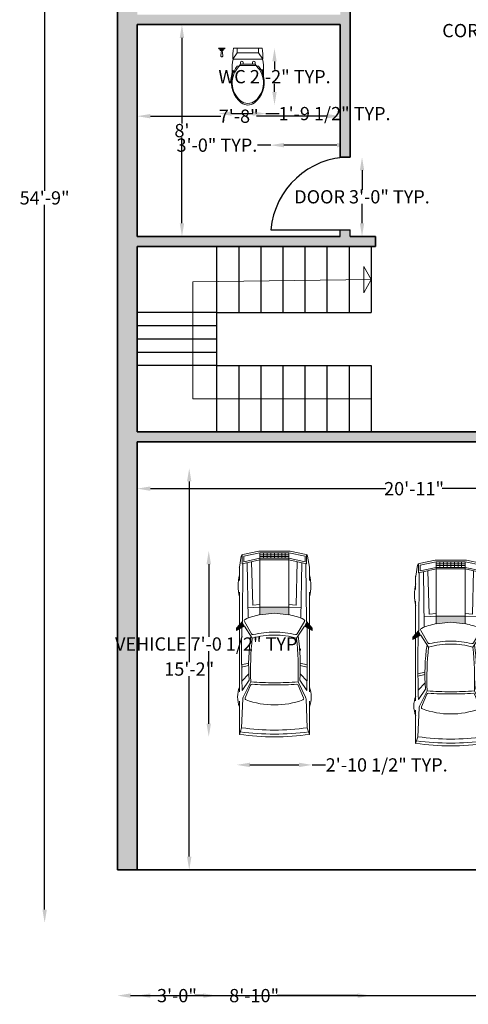
# Model space of a CAD drawing. Units: inches. Extents: x 2490 to 2996, y 1528 to 2269.
# Tile 1 of 4: x 2490 to 2693, y 1533 to 1979. Entities that reach past the tile are written whole.
import ezdxf

# ---------------------------------------------------------------- set-up
doc = ezdxf.new("R2010")
doc.units = ezdxf.units.IN
for name, color, linetype, lineweight in [('A-ANNO-DIMS', 2, 'Continuous', 18), ('A-DOOR', 4, 'Continuous', 25), ('A-EQPM-VEHL', 9, 'Continuous', 18), ('A-FLOR-STRS', 7, 'Continuous', 25), ('A-WALL', 7, 'Continuous', 35)]:
    doc.layers.add(name, color=color, linetype=linetype, lineweight=lineweight)
for name, color, linetype, lineweight, true_color in [('A-ANNO-SYMB', 244, 'Continuous', 18, 0x991b1e), ('A-FLOR-FIXT', 244, 'Continuous', 18, 0x991b1e), ('A-WALL-PATT', 85, 'Continuous', 13, 0x58ba48)]:
    doc.layers.add(name, color=color, linetype=linetype, lineweight=lineweight, true_color=true_color)
doc.styles.add('ATTR', font='romans.shx', dxfattribs={"width": 0.8, "height": 1.114828})
doc.styles.get("Standard").update_dxf_attribs({"font": 'arial.ttf'})
doc.dimstyles.get("Standard").update_dxf_attribs({"dimtxt": 6, "dimasz": 6, "dimexe": 0.18, "dimexo": 0.0625, "dimgap": 0.09, "dimtad": 0, "dimtih": 1, "dimtoh": 1, "dimdec": 4, "dimzin": 0, "dimdsep": 46, "dimlunit": 4, "dimtxsty": 'Standard', "dimcen": 0.09, "dimse1": 1, "dimse2": 1, "dimadec": 0, "dimazin": 0, "dimtfac": 1, "dimtdec": 4, "dimtofl": 0, "dimtmove": 0, "dimatfit": 3, "dimfxl": 1, "dimtolj": 1, "dimtzin": 0, "dimarcsym": 0})

# ---------------------------------------------------------------- blocks, each defined once
blk = doc.blocks.new('A$C682073C8')
for p, q in [((-2.78, 0.282), (-2.724, 0.571)), ((-2.69, 0.555), (-2.752, 0.263)), ((-2.554, 0.581), (-2.72, 0.581)), ((-2.694, 0.6), (-2.493, 0.633)), ((-2.59, 0.555), (-2.69, 0.555)), ((-2.59, 0.555), (-2.652, 0.263)), ((-2.554, 0.581), (-2.622, 0.263)), ((-2.557, 0.57), (-1.51, 0.58)), ((-2.251, 0.635), (-2.478, 0.635)), ((-1.445, 0.635), (-2.04, 0.635)), ((-1.51, 0.58), (-1.388, 0.684)), ((-1.286, 0.414), (-1.508, 0.544)), ((-1.428, 0.543), (-1.348, 0.684)), ((-1.209, 0.401), (-1.428, 0.543)), ((-1.388, 0.684), (-1.348, 0.684)), ((-0.237, 0.635), (-1.376, 0.635)), ((-0.755, 0.467), (-0.727, 0.593)), ((-0.714, 0.467), (-0.686, 0.593)), ((-0.432, 0.589), (-0.565, 0.464)), ((-0.451, 0.457), (-0.263, 0.585)), ((-0.142, 0.564), (-0.42, 0.428)), ((0.411, 0.593), (-0.11, 0.572)), ((0.532, 0.635), (-0.072, 0.635)), ((0.532, 0.635), (0.411, 0.593)), ((-1.805, 0.393), (-2.59, 0.413)), ((-1.57, 0.478), (-2.572, 0.496)), ((-1.818, 0.263), (-1.805, 0.393)), ((-1.771, 0.263), (-1.758, 0.481)), ((-0.361, 0.431), (-0.128, 0.528)), ((-2.781, 0), (-2.781, 0.273)), ((-2.752, 0.263), (-2.752, 0)), ((-1.633, 0.263), (-2.752, 0.263)), ((-2.652, 0.197), (-2.752, 0.197)), ((-2.718, 0.263), (-2.718, 0)), ((-2.685, 0.263), (-2.685, 0)), ((-2.652, 0.263), (-2.652, 0)), ((-2.622, 0.263), (-2.622, 0)), ((-1.771, 0.263), (-1.771, 0)), ((-1.633, 0.263), (-1.659, 0)), ((-2.781, 0), (-2.781, -0.273)), ((-2.652, 0.132), (-2.752, 0.132)), ((-2.652, 0.066), (-2.752, 0.066)), ((-2.652, 0), (-2.752, 0)), ((-2.752, -0.263), (-2.752, 0)), ((-2.718, -0.263), (-2.718, 0)), ((-2.685, -0.263), (-2.685, 0)), ((-2.652, -0.263), (-2.652, 0)), ((-2.622, -0.263), (-2.622, 0)), ((-1.771, -0.263), (-1.771, 0)), ((-1.659, 0), (-1.633, -0.263)), ((-2.652, -0.066), (-2.752, -0.066)), ((-2.652, -0.132), (-2.752, -0.132)), ((-2.78, -0.282), (-2.724, -0.571)), ((-2.652, -0.197), (-2.752, -0.197)), ((-1.633, -0.263), (-2.752, -0.263)), ((-2.69, -0.555), (-2.752, -0.263)), ((-2.59, -0.555), (-2.652, -0.263)), ((-2.554, -0.581), (-2.622, -0.263)), ((-1.818, -0.263), (-1.805, -0.393)), ((-1.771, -0.263), (-1.758, -0.481)), ((-1.805, -0.393), (-2.59, -0.413)), ((-1.57, -0.478), (-2.572, -0.496)), ((-1.286, -0.414), (-1.508, -0.544)), ((-1.209, -0.401), (-1.428, -0.543)), ((-0.755, -0.467), (-0.727, -0.593)), ((-0.714, -0.467), (-0.686, -0.593)), ((-0.432, -0.589), (-0.565, -0.464)), ((-0.451, -0.457), (-0.263, -0.585)), ((-0.142, -0.564), (-0.42, -0.428)), ((-0.361, -0.431), (-0.128, -0.528)), ((-2.554, -0.581), (-2.72, -0.581)), ((-2.694, -0.6), (-2.493, -0.633)), ((-2.59, -0.555), (-2.69, -0.555)), ((-2.557, -0.57), (-1.51, -0.58)), ((-2.251, -0.635), (-2.478, -0.635)), ((-1.445, -0.635), (-2.04, -0.635)), ((-1.51, -0.58), (-1.388, -0.684)), ((-1.428, -0.543), (-1.348, -0.684)), ((-1.388, -0.684), (-1.348, -0.684)), ((-0.237, -0.635), (-1.376, -0.635)), ((0.411, -0.593), (-0.11, -0.572)), ((0.532, -0.635), (-0.072, -0.635)), ((0.532, -0.635), (0.411, -0.593))]:
    blk.add_line(p, q)
for centre, radius, start, end in [((-2.688, 0.564), 0.0366, 99.5555, 168.9219), ((-2.478, 0.542), 0.0932, 90, 99.5555), ((-2.154, -0.189), 0.847, 76.4679, 103.5321), ((-1.522, 0.52), 0.0277, 59.6014, 156.2323), ((-0.97, -26.413), 27.007, 88.4985, 90.9138), ((-0.146, 0.162), 0.505, 69.2613, 110.7387), ((-0.106, 0.49), 0.0817, 92.3222, 116.0777), ((-3.642, 0), 4.096, 360, 8.3245), ((-4.512, 0), 5.038, 360, 7.0662), ((-3.75, 0), 4.328, 360, 8.4328), ((-0.341, 0), 1.319, 156.2323, 168.4871), ((0.324, 0), 1.642, 166.5017, 180), ((-1.3, 0.39), 0.0277, 346.5017, 59.6014), ((0.222, 0), 1.487, 164.3473, 180), ((-0.728, -3.189), 3.656, 85.6618, 98.2609), ((-0.642, -4.704), 5.136, 87.5218, 96.3432), ((-5.551, 0), 5.149, 360, 4.7655), ((-0.35, 0.407), 0.0264, 112.6283, 183.982), ((-6.195, 0), 5.833, 360, 3.982), ((-0.118, 0.504), 0.0264, 20.6689, 112.6283), ((-1.453, 0), 1.453, 360, 20.6689), ((-2.736, 0.273), 0.045, 168.9219, 180), ((0.324, 0), 1.642, 180, 193.4983), ((0.222, 0), 1.487, 180, 195.6527), ((-5.551, 0), 5.149, 355.2345, 360), ((-6.195, 0), 5.833, 356.018, 360), ((-1.453, 0), 1.453, 339.3311, 360), ((-3.642, 0), 4.096, 351.6755, 360), ((-4.512, 0), 5.038, 352.9338, 360), ((-3.75, 0), 4.328, 351.5672, 360), ((-2.736, -0.273), 0.045, 180, 191.0781), ((-0.341, 0), 1.319, 191.5129, 203.7677), ((-1.522, -0.52), 0.0277, 203.7677, 300.3986), ((-1.3, -0.39), 0.0277, 300.3986, 13.4983), ((-0.728, 3.189), 3.656, 261.7391, 274.3382), ((-0.642, 4.704), 5.136, 263.6568, 272.4781), ((-0.35, -0.407), 0.0264, 176.018, 247.3717), ((-0.118, -0.504), 0.0264, 247.3717, 339.3311), ((-2.688, -0.564), 0.0366, 191.0781, 260.4445), ((-2.478, -0.542), 0.0932, 260.4445, 270), ((-2.154, 0.189), 0.847, 256.4679, 283.5321), ((-0.97, 26.413), 27.007, 269.0862, 271.5015), ((-0.146, -0.162), 0.505, 249.2613, 290.7387), ((-0.106, -0.49), 0.0817, 243.9223, 267.6778)]:
    blk.add_arc(centre, radius, start, end)
for points in [[(-1.428, 0.543), (-1.51, 0.58), (-1.348, 0.684), (-1.388, 0.684)], [(-1.633, 0.263), (-1.659, 0), (-1.771, 0.263), (-1.771, -0.263)], [(-1.659, 0), (-1.633, -0.263), (-1.771, -0.263)], [(-1.428, -0.543), (-1.51, -0.58), (-1.348, -0.684), (-1.388, -0.684)]]:
    blk.add_solid(points)
at = {"style": 'ATTR', "width": 0.8, "flags": 9}
blk.add_attdef('ESTCODE', (-2.781, 0), '', height=0.00071, rotation=180, dxfattribs=at)
blk = doc.blocks.new('*D16')
at = {"layer": 'A-ANNO-DIMS', "color": 0, "lineweight": -2, "transparency": 16777216}
for p, q in [((2563.55, 1971.13), (2563.55, 1932.29)), ((2563.55, 1887.13), (2563.55, 1925.98))]:
    blk.add_line(p, q, dxfattribs=at)
at = {"layer": 'A-ANNO-DIMS', "color": 0, "transparency": 16777216}
for points in [[(2562.55, 1971.13), (2564.55, 1971.13), (2563.55, 1977.13)], [(2562.55, 1887.13), (2564.55, 1887.13), (2563.55, 1881.13)]]:
    blk.add_solid(points, dxfattribs=at)
at = {"layer": 'Defpoints', "color": 0, "transparency": 16777216}
for p in [(2543.28, 1977.13), (2543.28, 1881.13), (2563.55, 1881.13)]:
    blk.add_point(p, dxfattribs=at)
at = {"layer": 'A-ANNO-DIMS', "color": 0, "transparency": 16777216, "insert": (2563.55, 1929.13), "char_height": 6, "attachment_point": 5}
blk.add_mtext("\\A1;8'", dxfattribs=at)
blk = doc.blocks.new('*D17')
at = {"layer": 'A-ANNO-DIMS', "color": 0, "lineweight": -2, "transparency": 16777216}
for p, q in [((2549.28, 1935.65), (2581.24, 1935.65)), ((2629.28, 1935.65), (2597.32, 1935.65))]:
    blk.add_line(p, q, dxfattribs=at)
at = {"layer": 'A-ANNO-DIMS', "color": 0, "transparency": 16777216}
for points in [[(2549.28, 1936.65), (2549.28, 1934.65), (2543.28, 1935.65)], [(2629.28, 1936.65), (2629.28, 1934.65), (2635.28, 1935.65)]]:
    blk.add_solid(points, dxfattribs=at)
at = {"layer": 'Defpoints', "color": 0, "transparency": 16777216}
for p in [(2543.28, 1977.13), (2635.28, 1977.13), (2635.28, 1935.65)]:
    blk.add_point(p, dxfattribs=at)
at = {"layer": 'A-ANNO-DIMS', "color": 0, "transparency": 16777216, "insert": (2589.28, 1935.65), "char_height": 6, "attachment_point": 5}
blk.add_mtext('\\A1;7\'-8"', dxfattribs=at)
blk = doc.blocks.new('*D18')
at = {"layer": 'A-ANNO-DIMS', "color": 0, "lineweight": -2, "transparency": 16777216}
for p, q in [((2566.85, 1770.13), (2566.85, 1688.29)), ((2566.85, 1600.13), (2566.85, 1681.98))]:
    blk.add_line(p, q, dxfattribs=at)
at = {"layer": 'A-ANNO-DIMS', "color": 0, "transparency": 16777216}
for points in [[(2565.85, 1770.13), (2567.85, 1770.13), (2566.85, 1776.13)], [(2565.85, 1600.13), (2567.85, 1600.13), (2566.85, 1594.13)]]:
    blk.add_solid(points, dxfattribs=at)
at = {"layer": 'Defpoints', "color": 0, "transparency": 16777216}
for p in [(2543.28, 1776.13), (2543.28, 1594.13), (2566.85, 1594.13)]:
    blk.add_point(p, dxfattribs=at)
at = {"layer": 'A-ANNO-DIMS', "color": 0, "transparency": 16777216, "insert": (2566.85, 1685.13), "char_height": 6, "attachment_point": 5}
blk.add_mtext('\\A1;15\'-2"', dxfattribs=at)
blk = doc.blocks.new('*D19')
at = {"layer": 'A-ANNO-DIMS', "color": 0, "lineweight": -2, "transparency": 16777216}
for p, q in [((2549.28, 1766.88), (2656, 1766.88)), ((2788.28, 1766.88), (2681.56, 1766.88))]:
    blk.add_line(p, q, dxfattribs=at)
at = {"layer": 'A-ANNO-DIMS', "color": 0, "transparency": 16777216}
for points in [[(2549.28, 1767.88), (2549.28, 1765.88), (2543.28, 1766.88)], [(2788.28, 1767.88), (2788.28, 1765.88), (2794.28, 1766.88)]]:
    blk.add_solid(points, dxfattribs=at)
at = {"layer": 'Defpoints', "color": 0, "transparency": 16777216}
for p in [(2794.28, 1766.88), (2543.28, 1759.76), (2794.28, 1759.76)]:
    blk.add_point(p, dxfattribs=at)
at = {"layer": 'A-ANNO-DIMS', "color": 0, "transparency": 16777216, "insert": (2668.78, 1766.88), "char_height": 6, "attachment_point": 5}
blk.add_mtext('\\A1;20\'-11"', dxfattribs=at)
blk = doc.blocks.new('WC-PLAN')
for p, q in [((9.57, 17.88), (9.93, 18.54)), ((9.93, 18.54), (9.93, 19.26)), ((11.22, 18.54), (9.93, 18.54)), ((11.22, 19.26), (11.22, 18.54)), ((13.29, 18.54), (11.22, 18.54)), ((13.29, 18.54), (15.36, 18.54)), ((15.36, 19.26), (15.36, 18.54)), ((15.36, 18.54), (16.65, 18.54)), ((16.65, 18.54), (16.65, 19.26)), ((17.01, 17.88), (16.65, 18.54))]:
    blk.add_line(p, q)
for points in [[(2.96, 25.75), (0, 25.75)], [(2.78, 25.55), (0.18, 25.55)], [(2.16, 25.2), (0.8, 25.2)], [(0.8, 25.2), (0.8, 24.77), (1.28, 24.77)], [(1.15, 25.2), (1.15, 24.77)], [(1.28, 24.77), (1.71, 24.77)], [(1.71, 24.77), (2.14, 24.77), (2.16, 25.2)], [(1.84, 25.2), (1.84, 24.77)], [(6.49, 20.79), (8.51, 23.63), (8.51, 25.75)], [(19.81, 25.75), (6.76, 25.75)], [(8.51, 23.63), (13.29, 23.63)], [(18.06, 23.63), (13.29, 23.63)], [(20.09, 20.79), (18.06, 23.63), (18.06, 25.75)], [(6.61, 20.79), (13.29, 20.79)], [(19.96, 20.79), (13.29, 20.79)]]:
    blk.add_lwpolyline(points)
for points in [[(0.8, 25.2, -0.158381), (0, 25.75, 2.932383)], [(1.28, 24.75), (1.02, 22.39, 0.482607), (1.52, 21.9, -0.547905)], [(1.71, 24.75), (1.97, 22.39, -0.482607), (1.47, 21.9, 0.547905)], [(2.16, 25.2, 0.158381), (2.96, 25.75, -2.932383)], [(6.76, 25.75, 0.056711), (6.49, 20.79), (6.61, 20.79)], [(19.81, 25.75, -0.056711), (20.09, 20.79), (19.96, 20.79)], [(6.61, 20.78, 0.052121), (6.14, 15.38), (6.14, 13.01, 0.14456)], [(9.57, 17.88, 0.008985), (9.29, 17.61, 0.182634)], [(13.29, 17.88), (9.57, 17.88, 0.008985)], [(13.29, 17.88), (17.01, 17.88, -0.444938)], [(17.01, 17.88, -0.008985), (17.28, 17.61, -0.182634)], [(19.96, 20.78, -0.052121), (20.43, 15.38), (20.43, 13.01, -0.14456)], [(8.4, 17.61, 0.11024), (6.14, 13.01, 0.16845)], [(9.29, 17.61, 0.434217), (9.93, 1.97, 0.182634), (13.29, 0.75, 2.693815)], [(9.29, 17.61), (8.4, 17.61, 0.416606)], [(17.28, 17.61, -0.434217), (16.65, 1.97, -0.182634), (13.29, 0.75, -2.693815)], [(17.28, 17.61), (18.18, 17.61, -0.416606)], [(18.18, 17.61, -0.11024), (20.43, 13.01, -0.16845)], [(6.14, 13.01, 0.292914), (10.29, 1.04, 0.16845), (13.29, 0, 2.883082)], [(20.43, 13.01, -0.292914), (16.29, 1.04, -0.16845), (13.29, 0, -2.883082)]]:
    blk.add_lwpolyline(points, format="xyb")
for centre in [(10.57, 19.26), (16, 19.26)]:
    blk.add_arc(centre, 0.645, 0, 180)
blk = doc.blocks.new('DOOR-SINGLE-36IN')
for p, q in [((0, 36), (0, 4.5)), ((3, 35.88), (3, 0)), ((0, 4.5), (3, 4.5)), ((0, 0), (3, 0))]:
    blk.add_line(p, q)
blk.add_arc((0, 0), 36, 0, 85.2198)
blk = doc.blocks.new('*D32')
at = {"layer": 'A-ANNO-DIMS', "color": 0, "lineweight": -2, "transparency": 16777216}
for p, q in [((2605.51, 1960.45), (2605.51, 1956.76)), ((2605.51, 1946.69), (2605.51, 1950.38))]:
    blk.add_line(p, q, dxfattribs=at)
at = {"layer": 'A-ANNO-DIMS', "color": 0, "transparency": 16777216}
for points in [[(2604.51, 1960.45), (2606.51, 1960.45), (2605.51, 1966.45)], [(2604.51, 1946.69), (2606.51, 1946.69), (2605.51, 1940.69)]]:
    blk.add_solid(points, dxfattribs=at)
at = {"layer": 'Defpoints', "color": 0, "transparency": 16777216}
for p in [(2601.65, 1966.45), (2605.51, 1966.45), (2601.65, 1940.69)]:
    blk.add_point(p, dxfattribs=at)
at = {"layer": 'A-ANNO-DIMS', "color": 0, "transparency": 16777216, "insert": (2605.51, 1953.57), "char_height": 6, "attachment_point": 5}
blk.add_mtext('\\A1;WC 2\'-2" TYP.', dxfattribs=at)
blk = doc.blocks.new('*D33')
at = {"layer": 'A-ANNO-DIMS', "color": 0, "lineweight": -2, "transparency": 16777216}
for p, q in [((2586.14, 1936.83), (2595.65, 1936.83)), ((2601.65, 1936.83), (2607.65, 1936.83))]:
    blk.add_line(p, q, dxfattribs=at)
at = {"layer": 'A-ANNO-DIMS', "color": 0, "transparency": 16777216}
for points in [[(2586.14, 1937.83), (2586.14, 1935.83), (2580.14, 1936.83)], [(2595.65, 1937.83), (2595.65, 1935.83), (2601.65, 1936.83)]]:
    blk.add_solid(points, dxfattribs=at)
at = {"layer": 'Defpoints', "color": 0, "transparency": 16777216}
for p in [(2580.14, 1940.69), (2601.65, 1940.69), (2601.65, 1936.83)]:
    blk.add_point(p, dxfattribs=at)
at = {"layer": 'A-ANNO-DIMS', "color": 0, "transparency": 16777216, "insert": (2632.73, 1936.83), "char_height": 6, "attachment_point": 5}
blk.add_mtext('\\A1;1\'-9 1/2" TYP.', dxfattribs=at)
blk = doc.blocks.new('*D34')
at = {"layer": 'A-ANNO-DIMS', "color": 0, "lineweight": -2, "transparency": 16777216}
for p, q in [((2645.18, 1911.13), (2645.18, 1902.33)), ((2645.18, 1887.13), (2645.18, 1895.94))]:
    blk.add_line(p, q, dxfattribs=at)
at = {"layer": 'A-ANNO-DIMS', "color": 0, "transparency": 16777216}
for points in [[(2644.18, 1911.13), (2646.18, 1911.13), (2645.18, 1917.13)], [(2644.18, 1887.13), (2646.18, 1887.13), (2645.18, 1881.13)]]:
    blk.add_solid(points, dxfattribs=at)
at = {"layer": 'Defpoints', "color": 0, "transparency": 16777216}
for p in [(2639.78, 1917.13), (2645.18, 1917.13), (2639.78, 1881.13)]:
    blk.add_point(p, dxfattribs=at)
at = {"layer": 'A-ANNO-DIMS', "color": 0, "transparency": 16777216, "insert": (2645.18, 1899.13), "char_height": 6, "attachment_point": 5}
blk.add_mtext('\\A1;DOOR 3\'-0" TYP.', dxfattribs=at)
blk = doc.blocks.new('*D35')
at = {"layer": 'A-ANNO-DIMS', "color": 0, "lineweight": -2, "transparency": 16777216}
for p, q in [((2603.78, 1922.53), (2597.78, 1922.53)), ((2633.78, 1922.53), (2609.78, 1922.53))]:
    blk.add_line(p, q, dxfattribs=at)
at = {"layer": 'A-ANNO-DIMS', "color": 0, "transparency": 16777216}
for points in [[(2609.78, 1923.53), (2609.78, 1921.53), (2603.78, 1922.53)], [(2633.78, 1923.53), (2633.78, 1921.53), (2639.78, 1922.53)]]:
    blk.add_solid(points, dxfattribs=at)
at = {"layer": 'Defpoints', "color": 0, "transparency": 16777216}
for p in [(2603.78, 1922.53), (2603.78, 1917.13), (2639.78, 1917.13)]:
    blk.add_point(p, dxfattribs=at)
at = {"layer": 'A-ANNO-DIMS', "color": 0, "transparency": 16777216, "insert": (2579.4, 1922.53), "char_height": 6, "attachment_point": 5}
blk.add_mtext('\\A1;3\'-0" TYP.', dxfattribs=at)
blk = doc.blocks.new('*D38')
at = {"layer": 'A-ANNO-DIMS', "color": 0, "lineweight": -2, "transparency": 16777216}
for p, q in [((2575.7, 1732.64), (2575.7, 1699.69)), ((2575.7, 1660.35), (2575.7, 1693.3))]:
    blk.add_line(p, q, dxfattribs=at)
at = {"layer": 'A-ANNO-DIMS', "color": 0, "transparency": 16777216}
for points in [[(2574.7, 1732.64), (2576.7, 1732.64), (2575.7, 1738.64)], [(2574.7, 1660.35), (2576.7, 1660.35), (2575.7, 1654.35)]]:
    blk.add_solid(points, dxfattribs=at)
at = {"layer": 'Defpoints', "color": 0, "transparency": 16777216}
for p in [(2588.35, 1738.64), (2575.7, 1654.35), (2588.35, 1654.35)]:
    blk.add_point(p, dxfattribs=at)
at = {"layer": 'A-ANNO-DIMS', "color": 0, "transparency": 16777216, "insert": (2575.7, 1696.49), "char_height": 6, "attachment_point": 5}
blk.add_mtext('\\A1;VEHICLE 7\'-0 1/2" TYP.', dxfattribs=at)
blk = doc.blocks.new('*D39')
at = {"layer": 'A-ANNO-DIMS', "color": 0, "lineweight": -2, "transparency": 16777216}
for p, q in [((2594.35, 1641.7), (2616.61, 1641.7)), ((2622.61, 1641.7), (2628.61, 1641.7))]:
    blk.add_line(p, q, dxfattribs=at)
at = {"layer": 'A-ANNO-DIMS', "color": 0, "transparency": 16777216}
for points in [[(2594.35, 1642.7), (2594.35, 1640.7), (2588.35, 1641.7)], [(2616.61, 1642.7), (2616.61, 1640.7), (2622.61, 1641.7)]]:
    blk.add_solid(points, dxfattribs=at)
at = {"layer": 'Defpoints', "color": 0, "transparency": 16777216}
for p in [(2588.35, 1654.35), (2622.61, 1654.35), (2622.61, 1641.7)]:
    blk.add_point(p, dxfattribs=at)
at = {"layer": 'A-ANNO-DIMS', "color": 0, "transparency": 16777216, "insert": (2656.36, 1641.7), "char_height": 6, "attachment_point": 5}
blk.add_mtext('\\A1;2\'-10 1/2" TYP.', dxfattribs=at)
blk = doc.blocks.new('*D40')
at = {"layer": 'A-ANNO-DIMS', "color": 0, "lineweight": -2, "transparency": 16777216}
for p, q in [((2801.71, 1974.44), (2795.71, 1974.44)), ((2821.13, 1974.44), (2807.71, 1974.44))]:
    blk.add_line(p, q, dxfattribs=at)
at = {"layer": 'A-ANNO-DIMS', "color": 0, "transparency": 16777216}
for points in [[(2807.71, 1975.44), (2807.71, 1973.44), (2801.71, 1974.44)], [(2821.13, 1975.44), (2821.13, 1973.44), (2827.13, 1974.44)]]:
    blk.add_solid(points, dxfattribs=at)
at = {"layer": 'Defpoints', "color": 0, "transparency": 16777216}
for p in [(2801.71, 1974.44), (2801.71, 1970.63), (2827.13, 1970.63)]:
    blk.add_point(p, dxfattribs=at)
at = {"layer": 'A-ANNO-DIMS', "color": 0, "transparency": 16777216, "insert": (2736.85, 1974.44), "char_height": 6, "attachment_point": 5}
blk.add_mtext('\\A1;CORNER CHAIR 2\'-1 1/2" TYP.', dxfattribs=at)
blk = doc.blocks.new('*D46')
at = {"layer": 'A-ANNO-DIMS', "color": 0, "lineweight": -2, "transparency": 16777216}
for p, q in [((2540.28, 1537.16), (2732.39, 1537.16)), ((2945.28, 1537.16), (2753.17, 1537.16))]:
    blk.add_line(p, q, dxfattribs=at)
at = {"layer": 'A-ANNO-DIMS', "color": 0, "transparency": 16777216}
for points in [[(2540.28, 1538.16), (2540.28, 1536.16), (2534.28, 1537.16)], [(2945.28, 1538.16), (2945.28, 1536.16), (2951.28, 1537.16)]]:
    blk.add_solid(points, dxfattribs=at)
at = {"layer": 'Defpoints', "color": 0, "transparency": 16777216}
for p in [(2951.28, 1600.13), (2534.28, 1594.13), (2951.28, 1537.16)]:
    blk.add_point(p, dxfattribs=at)
at = {"layer": 'A-ANNO-DIMS', "color": 0, "transparency": 16777216, "insert": (2742.78, 1537.16), "char_height": 6, "attachment_point": 5}
blk.add_mtext('\\A1;34\'-9"', dxfattribs=at)
blk = doc.blocks.new('*D47')
at = {"layer": 'A-ANNO-DIMS', "color": 0, "lineweight": -2, "transparency": 16777216}
for p, q in [((2501.3, 2221.13), (2501.3, 1901.79)), ((2501.3, 1576.13), (2501.3, 1895.48))]:
    blk.add_line(p, q, dxfattribs=at)
at = {"layer": 'A-ANNO-DIMS', "color": 0, "transparency": 16777216}
for points in [[(2500.3, 2221.13), (2502.3, 2221.13), (2501.3, 2227.13)], [(2500.3, 1576.13), (2502.3, 1576.13), (2501.3, 1570.13)]]:
    blk.add_solid(points, dxfattribs=at)
at = {"layer": 'Defpoints', "color": 0, "transparency": 16777216}
for p in [(2501.3, 2227.13), (2534.28, 2227.13), (2758.28, 1570.13)]:
    blk.add_point(p, dxfattribs=at)
at = {"layer": 'A-ANNO-DIMS', "color": 0, "transparency": 16777216, "insert": (2501.3, 1898.63), "char_height": 6, "attachment_point": 5}
blk.add_mtext('\\A1;54\'-9"', dxfattribs=at)
blk = doc.blocks.new('*D50')
at = {"layer": 'A-ANNO-DIMS', "color": 0, "lineweight": -2, "transparency": 16777216}
for p, q in [((2984.25, 1870.63), (2984.25, 1837.79)), ((2984.25, 1798.63), (2984.25, 1831.48))]:
    blk.add_line(p, q, dxfattribs=at)
at = {"layer": 'A-ANNO-DIMS', "color": 0, "transparency": 16777216}
for points in [[(2983.25, 1870.63), (2985.25, 1870.63), (2984.25, 1876.63)], [(2983.25, 1798.63), (2985.25, 1798.63), (2984.25, 1792.63)]]:
    blk.add_solid(points, dxfattribs=at)
at = {"layer": 'Defpoints', "color": 0, "transparency": 16777216}
for p in [(2649.28, 1876.63), (2984.25, 1876.63), (2649.28, 1792.63)]:
    blk.add_point(p, dxfattribs=at)
at = {"layer": 'A-ANNO-DIMS', "color": 0, "transparency": 16777216, "insert": (2984.25, 1834.63), "char_height": 6, "attachment_point": 5}
blk.add_mtext('\\A1;7\'-0"', dxfattribs=at)
blk = doc.blocks.new('*D51')
at = {"layer": 'A-ANNO-DIMS', "color": 0, "lineweight": -2, "transparency": 16777216}
for p, q in [((2549.28, 1537.16), (2585.88, 1537.16)), ((2643.28, 1537.16), (2606.68, 1537.16))]:
    blk.add_line(p, q, dxfattribs=at)
at = {"layer": 'A-ANNO-DIMS', "color": 0, "transparency": 16777216}
for points in [[(2549.28, 1538.16), (2549.28, 1536.16), (2543.28, 1537.16)], [(2643.28, 1538.16), (2643.28, 1536.16), (2649.28, 1537.16)]]:
    blk.add_solid(points, dxfattribs=at)
at = {"layer": 'Defpoints', "color": 0, "transparency": 16777216}
for p in [(2543.28, 1792.63), (2649.28, 1792.63), (2649.28, 1537.16)]:
    blk.add_point(p, dxfattribs=at)
at = {"layer": 'A-ANNO-DIMS', "color": 0, "transparency": 16777216, "insert": (2596.28, 1537.16), "char_height": 6, "attachment_point": 5}
blk.add_mtext('\\A1;8\'-10"', dxfattribs=at)
blk = doc.blocks.new('*D52')
at = {"layer": 'A-ANNO-DIMS', "color": 0, "lineweight": -2, "transparency": 16777216}
for p, q in [((2984.25, 1816.63), (2984.25, 1810.79)), ((2984.25, 1798.63), (2984.25, 1804.48))]:
    blk.add_line(p, q, dxfattribs=at)
at = {"layer": 'A-ANNO-DIMS', "color": 0, "transparency": 16777216}
for points in [[(2983.25, 1816.63), (2985.25, 1816.63), (2984.25, 1822.63)], [(2983.25, 1798.63), (2985.25, 1798.63), (2984.25, 1792.63)]]:
    blk.add_solid(points, dxfattribs=at)
at = {"layer": 'Defpoints', "color": 0, "transparency": 16777216}
for p in [(2649.28, 1822.63), (2984.25, 1822.63), (2649.28, 1792.63)]:
    blk.add_point(p, dxfattribs=at)
at = {"layer": 'A-ANNO-DIMS', "color": 0, "transparency": 16777216, "insert": (2984.25, 1807.63), "char_height": 6, "attachment_point": 5}
blk.add_mtext('\\A1;2\'-6"', dxfattribs=at)
blk = doc.blocks.new('*D53')
at = {"layer": 'A-ANNO-DIMS', "color": 0, "lineweight": -2, "transparency": 16777216}
for p, q in [((2549.28, 1537.16), (2553.22, 1537.16)), ((2573.28, 1537.16), (2569.34, 1537.16))]:
    blk.add_line(p, q, dxfattribs=at)
at = {"layer": 'A-ANNO-DIMS', "color": 0, "transparency": 16777216}
for points in [[(2549.28, 1538.16), (2549.28, 1536.16), (2543.28, 1537.16)], [(2573.28, 1538.16), (2573.28, 1536.16), (2579.28, 1537.16)]]:
    blk.add_solid(points, dxfattribs=at)
at = {"layer": 'Defpoints', "color": 0, "transparency": 16777216}
for p in [(2543.28, 1822.63), (2579.28, 1822.63), (2579.28, 1537.16)]:
    blk.add_point(p, dxfattribs=at)
at = {"layer": 'A-ANNO-DIMS', "color": 0, "transparency": 16777216, "insert": (2561.28, 1537.16), "char_height": 6, "attachment_point": 5}
blk.add_mtext('\\A1;3\'-0"', dxfattribs=at)
blk = doc.blocks.new('*D54')
at = {"layer": 'A-ANNO-DIMS', "color": 0, "lineweight": -2, "transparency": 16777216}
for p, q in [((2633.28, 2260.11), (2627.28, 2260.11)), ((2655.28, 2260.11), (2661.28, 2260.11))]:
    blk.add_line(p, q, dxfattribs=at)
at = {"layer": 'A-ANNO-DIMS', "color": 0, "transparency": 16777216}
for points in [[(2633.28, 2261.11), (2633.28, 2259.11), (2639.28, 2260.11)], [(2655.28, 2261.11), (2655.28, 2259.11), (2649.28, 2260.11)]]:
    blk.add_solid(points, dxfattribs=at)
at = {"layer": 'Defpoints', "color": 0, "transparency": 16777216}
for p in [(2649.28, 2260.11), (2639.28, 1822.63), (2649.28, 1822.63)]:
    blk.add_point(p, dxfattribs=at)
at = {"layer": 'A-ANNO-DIMS', "color": 0, "transparency": 16777216, "insert": (2671.67, 2260.11), "char_height": 6, "attachment_point": 5}
blk.add_mtext('\\A1;0\'-10"', dxfattribs=at)

msp = doc.modelspace()

# ---------------------------------------------------------------- hatches: boundary and pattern name
at = {"layer": 'A-WALL-PATT'}
h = msp.add_hatch(color=256, dxfattribs=at)
h.dxf.hatch_style = 1
h.paths.add_polyline_path([(2951.27862, 2227.13248), (2534.27862, 2227.13248), (2534.27862, 1594.13248), (2543.27862, 1594.13248), (2543.27862, 1776.13248), (2543.27862, 1780.63248), (2543.27862, 1788.13248), (2639.77862, 1788.13248), (2722.27862, 1788.13248), (2722.27862, 1792.63248), (2639.77862, 1792.63248), (2543.27862, 1792.63248), (2543.27862, 1822.63248), (2543.27862, 1876.63248), (2639.77862, 1876.63248), (2651.27862, 1876.63248), (2651.27862, 1881.13248), (2639.77862, 1881.13248), (2639.77862, 1884.13248), (2635.27862, 1884.13248), (2635.27862, 1881.13248), (2603.77862, 1881.13248), (2543.27862, 1881.13248), (2543.27862, 1977.13248), (2635.27862, 1977.13248), (2635.27862, 1917.13248), (2639.77862, 1917.13248), (2639.77862, 2057.63248), (2651.27862, 2057.63248), (2651.27862, 2062.13248), (2635.27862, 2062.13248), (2635.27862, 2057.63248), (2635.27862, 1981.63248), (2543.27862, 1981.63248), (2543.27862, 2057.63248), (2605.27862, 2057.63248), (2605.27862, 2062.13248), (2543.27862, 2062.13248), (2543.27862, 2218.13248), (2687.27862, 2218.13248), (2687.27862, 2062.13248), (2684.27862, 2062.13248), (2684.27862, 2057.63248), (2687.27862, 2057.63248), (2691.77862, 2057.63248), (2694.77862, 2057.63248), (2694.77862, 2062.13248), (2691.77862, 2062.13248), (2691.77862, 2093.63248), (2691.77862, 2218.13248), (2823.77862, 2218.13248), (2823.77862, 2062.13248), (2727.77862, 2062.13248), (2727.77862, 2057.63248), (2828.27862, 2057.63248), (2831.27862, 2057.63248), (2831.27862, 2062.13248), (2828.27862, 2062.13248), (2828.27862, 2093.63248), (2828.27862, 2218.13248), (2942.27862, 2218.13248), (2942.27862, 2062.13248), (2864.27862, 2062.13248), (2864.27862, 2057.63248), (2942.27862, 2057.63248), (2942.27862, 1757.63248), (2834.77862, 1757.63248), (2834.77862, 1753.13248), (2942.27862, 1753.13248), (2942.27862, 1609.13248), (2798.77862, 1609.13248), (2798.77862, 1600.13248), (2951.27862, 1600.13248)])
h.paths.add_polyline_path([(2798.77862, 1753.13248), (2801.77862, 1753.13248), (2801.77862, 1757.63248), (2798.77862, 1757.63248), (2798.77862, 1780.63248), (2798.77862, 1792.63248), (2794.27862, 1792.63248), (2794.27862, 1788.13248), (2794.27862, 1776.13248), (2794.27862, 1757.63248), (2794.27862, 1594.13248), (2798.77862, 1594.13248)], flags=17)

# ---------------------------------------------------------------- linework, layer by layer
at = {"layer": 'A-ANNO-SYMB'}
for p, q in [((2645.97216, 1861.5925), (2645.97216, 1867.5925)), ((2645.97216, 1867.5925), (2645.97216, 1855.5925)), ((2649.27862, 1861.63248), (2645.97216, 1867.5925)), ((2568.52073, 1860.65597), (2649.27862, 1861.63248)), ((2568.52073, 1807.63248), (2568.52073, 1860.65597)), ((2645.97216, 1855.5925), (2649.27862, 1861.63248)), ((2649.27862, 1807.63248), (2568.52073, 1807.63248))]:
    msp.add_line(p, q, dxfattribs=at)
at = {"layer": 'A-FLOR-STRS'}
for p, q in [((2579.27862, 1876.63248), (2579.27862, 1792.63248)), ((2589.27862, 1876.63248), (2589.27862, 1846.63248)), ((2599.27862, 1876.63248), (2599.27862, 1846.63248)), ((2609.27862, 1876.63248), (2609.27862, 1846.63248)), ((2619.27862, 1876.63248), (2619.27862, 1846.63248)), ((2629.27862, 1876.63248), (2629.27862, 1846.63248)), ((2639.27862, 1876.63248), (2639.27862, 1846.63248)), ((2649.27862, 1876.63248), (2649.27862, 1846.63248)), ((2579.27862, 1846.63248), (2543.27862, 1846.63248)), ((2579.27862, 1846.63248), (2543.27862, 1846.63248)), ((2579.27862, 1846.63248), (2543.27862, 1846.63248)), ((2579.27862, 1846.63248), (2543.27862, 1846.63248)), ((2579.27862, 1846.63248), (2649.27862, 1846.63248)), ((2579.27862, 1840.63248), (2543.27862, 1840.63248)), ((2579.27862, 1834.63248), (2543.27862, 1834.63248)), ((2579.27862, 1828.63248), (2543.27862, 1828.63248)), ((2543.27862, 1792.63248), (2543.27862, 1822.63248)), ((2579.27862, 1822.63248), (2543.27862, 1822.63248)), ((2579.27862, 1822.63248), (2649.27862, 1822.63248)), ((2589.27862, 1822.63248), (2589.27862, 1792.63248)), ((2599.27862, 1822.63248), (2599.27862, 1792.63248)), ((2609.27862, 1822.63248), (2609.27862, 1792.63248)), ((2619.27862, 1822.63248), (2619.27862, 1792.63248)), ((2629.27862, 1822.63248), (2629.27862, 1792.63248)), ((2639.27862, 1822.63248), (2639.27862, 1792.63248)), ((2649.27862, 1822.63248), (2649.27862, 1792.63248))]:
    msp.add_line(p, q, dxfattribs=at)
at = {"layer": 'A-WALL'}
for p, q in [((2534.27862, 2227.13248), (2534.27862, 1594.13248)), ((2639.77862, 2057.63248), (2639.77862, 1917.13248)), ((2543.27862, 1977.13248), (2635.27862, 1977.13248)), ((2543.27862, 1977.13248), (2543.27862, 1881.13248)), ((2635.27862, 1977.13248), (2635.27862, 1917.13248)), ((2639.77862, 1917.13248), (2635.27862, 1917.13248)), ((2543.27862, 1881.13248), (2635.27862, 1881.13248)), ((2639.77862, 1881.13248), (2651.27862, 1881.13248)), ((2651.27862, 1881.13248), (2651.27862, 1876.63248)), ((2543.27862, 1876.63248), (2639.77862, 1876.63248)), ((2543.27862, 1876.63248), (2543.27862, 1792.63248)), ((2651.27862, 1876.63248), (2639.77862, 1876.63248)), ((2543.27862, 1792.63248), (2639.77862, 1792.63248)), ((2639.77862, 1792.63248), (2722.27862, 1792.63248)), ((2543.27862, 1788.13248), (2639.77862, 1788.13248)), ((2543.27862, 1788.13248), (2543.27862, 1780.63248)), ((2722.27862, 1788.13248), (2639.77862, 1788.13248)), ((2543.27862, 1780.63248), (2543.27862, 1776.13248)), ((2543.27862, 1776.13248), (2543.27862, 1594.13248)), ((2798.77862, 1594.13248), (2534.27862, 1594.13248))]:
    msp.add_line(p, q, dxfattribs=at)

# ---------------------------------------------------------------- block references
at = {"layer": 'A-DOOR', "rotation": 90.00000000000115}
msp.add_blockref('DOOR-SINGLE-36IN', (2639.7791, 1881.13285), dxfattribs=at)
at = {"layer": 'A-EQPM-VEHL', "xscale": 25.05891406784298, "yscale": 25.05891406784298, "zscale": 25.05891406784298, "rotation": 270}
for p in [(2605.47944, 1668.85101), (2685.40516, 1664.76968)]:
    msp.add_blockref('A$C682073C8', p, dxfattribs=at)
at = {"layer": 'A-FLOR-FIXT'}
msp.add_blockref('WC-PLAN', (2580.14, 1940.694), dxfattribs=at)

# ---------------------------------------------------------------- dimensions: what is measured, and where the dimension line sits
at = {"layer": 'A-ANNO-DIMS'}
for base, p1, p2, override, picture, middle in [((2649.27862, 2260.10748), (2639.27862, 1822.63248), (2649.27862, 1822.63248), {"dimdec": 1, "dimlfac": 1, "dimrnd": 0, "dimzin": 1, "dimdsep": 46, "dimlunit": 4, "dimfrac": 2}, '*D54', (2671.67422, 2260.10748)), ((2635.27862, 1935.64876), (2543.27862, 1977.13248), (2635.27862, 1977.13248), {"dimclrd": 0, "dimclre": 0, "dimclrt": 0}, '*D17', (2589.27862, 1935.64876)), ((2579.27862, 1537.15748), (2543.27862, 1822.63248), (2579.27862, 1822.63248), {"dimdec": 1, "dimlfac": 1, "dimrnd": 0, "dimzin": 1, "dimdsep": 46, "dimlunit": 4, "dimfrac": 2}, '*D53', (2561.27862, 1537.15748)), ((2649.27862, 1537.15748), (2543.27862, 1792.63248), (2649.27862, 1792.63248), {"dimdec": 1, "dimlfac": 1, "dimrnd": 0, "dimzin": 1, "dimdsep": 46, "dimlunit": 4, "dimfrac": 2}, '*D51', (2596.27862, 1537.15748)), ((2794.27862, 1766.88248), (2543.27862, 1759.76434), (2794.27862, 1759.76434), {"dimclrd": 0, "dimclre": 0, "dimclrt": 0}, '*D19', (2668.77862, 1766.88248)), ((2951.27862, 1537.15748), (2534.27862, 1594.13248), (2951.27862, 1600.13248), {"dimdec": 1, "dimlfac": 1, "dimrnd": 0, "dimzin": 1, "dimdsep": 46, "dimlunit": 4, "dimfrac": 2}, '*D46', (2742.77862, 1537.15748))]:
    dim = msp.add_linear_dim(base=base, p1=p1, p2=p2, dimstyle='Standard', override=override, dxfattribs=at)
    dim.commit()
    dim.dimension.update_dxf_attribs({"geometry": picture, "text_midpoint": middle})
for base, p1, p2, override, picture, middle in [((2501.30362, 2227.13248), (2758.27862, 1570.13248), (2534.27862, 2227.13248), {"dimdec": 1, "dimlfac": 1, "dimrnd": 0, "dimzin": 1, "dimdsep": 46, "dimlunit": 4, "dimfrac": 2}, '*D47', (2501.30362, 1898.63248)), ((2563.54928, 1881.13248), (2543.27862, 1977.13248), (2543.27862, 1881.13248), {"dimclrd": 0, "dimclre": 0, "dimclrt": 0}, '*D16', (2563.54928, 1929.13248)), ((2984.25362, 1876.63248), (2649.27862, 1792.63248), (2649.27862, 1876.63248), {"dimdec": 1, "dimlfac": 1, "dimrnd": 0, "dimzin": 1, "dimdsep": 46, "dimlunit": 4, "dimfrac": 2}, '*D50', (2984.25362, 1834.63248)), ((2984.25362, 1822.63248), (2649.27862, 1792.63248), (2649.27862, 1822.63248), {"dimdec": 1, "dimlfac": 1, "dimrnd": 0, "dimzin": 1, "dimdsep": 46, "dimlunit": 4, "dimfrac": 2}, '*D52', (2984.25362, 1807.63248)), ((2566.84558, 1594.13248), (2543.27862, 1776.13248), (2543.27862, 1594.13248), {"dimclrd": 0, "dimclre": 0, "dimclrt": 0}, '*D18', (2566.84558, 1685.13248))]:
    dim = msp.add_linear_dim(base=base, p1=p1, p2=p2, angle=90, dimstyle='Standard', override=override, dxfattribs=at)
    dim.commit()
    dim.dimension.update_dxf_attribs({"geometry": picture, "text_midpoint": middle})
for base, p1, p2, angle, text, picture, middle in [((2801.71476, 1974.44006), (2827.13382, 1970.6272), (2801.71476, 1970.6272), 180, 'CORNER CHAIR <> TYP.', '*D40', (2736.85259, 1974.44006)), ((2605.50816, 1966.44634), (2601.64524, 1940.69357), (2601.64524, 1966.44634), 90, 'WC <> TYP.', '*D32', (2605.50816, 1953.56995)), ((2603.77862, 1922.53248), (2639.77862, 1917.13248), (2603.77862, 1917.13248), 180, '<> TYP.', '*D35', (2579.40418, 1922.53248)), ((2645.17862, 1917.13248), (2639.77862, 1881.13248), (2639.77862, 1917.13248), 90, 'DOOR <> TYP.', '*D34', (2645.17862, 1899.13248)), ((2575.70344, 1654.34805), (2588.34714, 1738.63937), (2588.34714, 1654.34805), 270, 'VEHICLE <> TYP.', '*D38', (2575.70344, 1696.49371))]:
    dim = msp.add_linear_dim(base=base, p1=p1, p2=p2, angle=angle, text=text, dimstyle='Standard', override={"dimdec": 1, "dimlfac": 1, "dimrnd": 0, "dimzin": 1, "dimdsep": 46, "dimlunit": 4, "dimfrac": 2}, dxfattribs=at)
    dim.commit()
    dim.dimension.update_dxf_attribs({"geometry": picture, "text_midpoint": middle})
for base, p1, p2, picture, middle in [((2601.64524, 1936.83065), (2580.13964, 1940.69357), (2601.64524, 1940.69357), '*D33', (2632.72979, 1936.83065)), ((2622.61175, 1641.70435), (2588.34714, 1654.34805), (2622.61175, 1654.34805), '*D39', (2656.36069, 1641.70435))]:
    dim = msp.add_linear_dim(base=base, p1=p1, p2=p2, text='<> TYP.', dimstyle='Standard', override={"dimdec": 1, "dimlfac": 1, "dimrnd": 0, "dimzin": 1, "dimdsep": 46, "dimlunit": 4, "dimfrac": 2}, dxfattribs=at)
    dim.commit()
    dim.dimension.update_dxf_attribs({"geometry": picture, "text_midpoint": middle})

doc.saveas('drawing.dxf')
